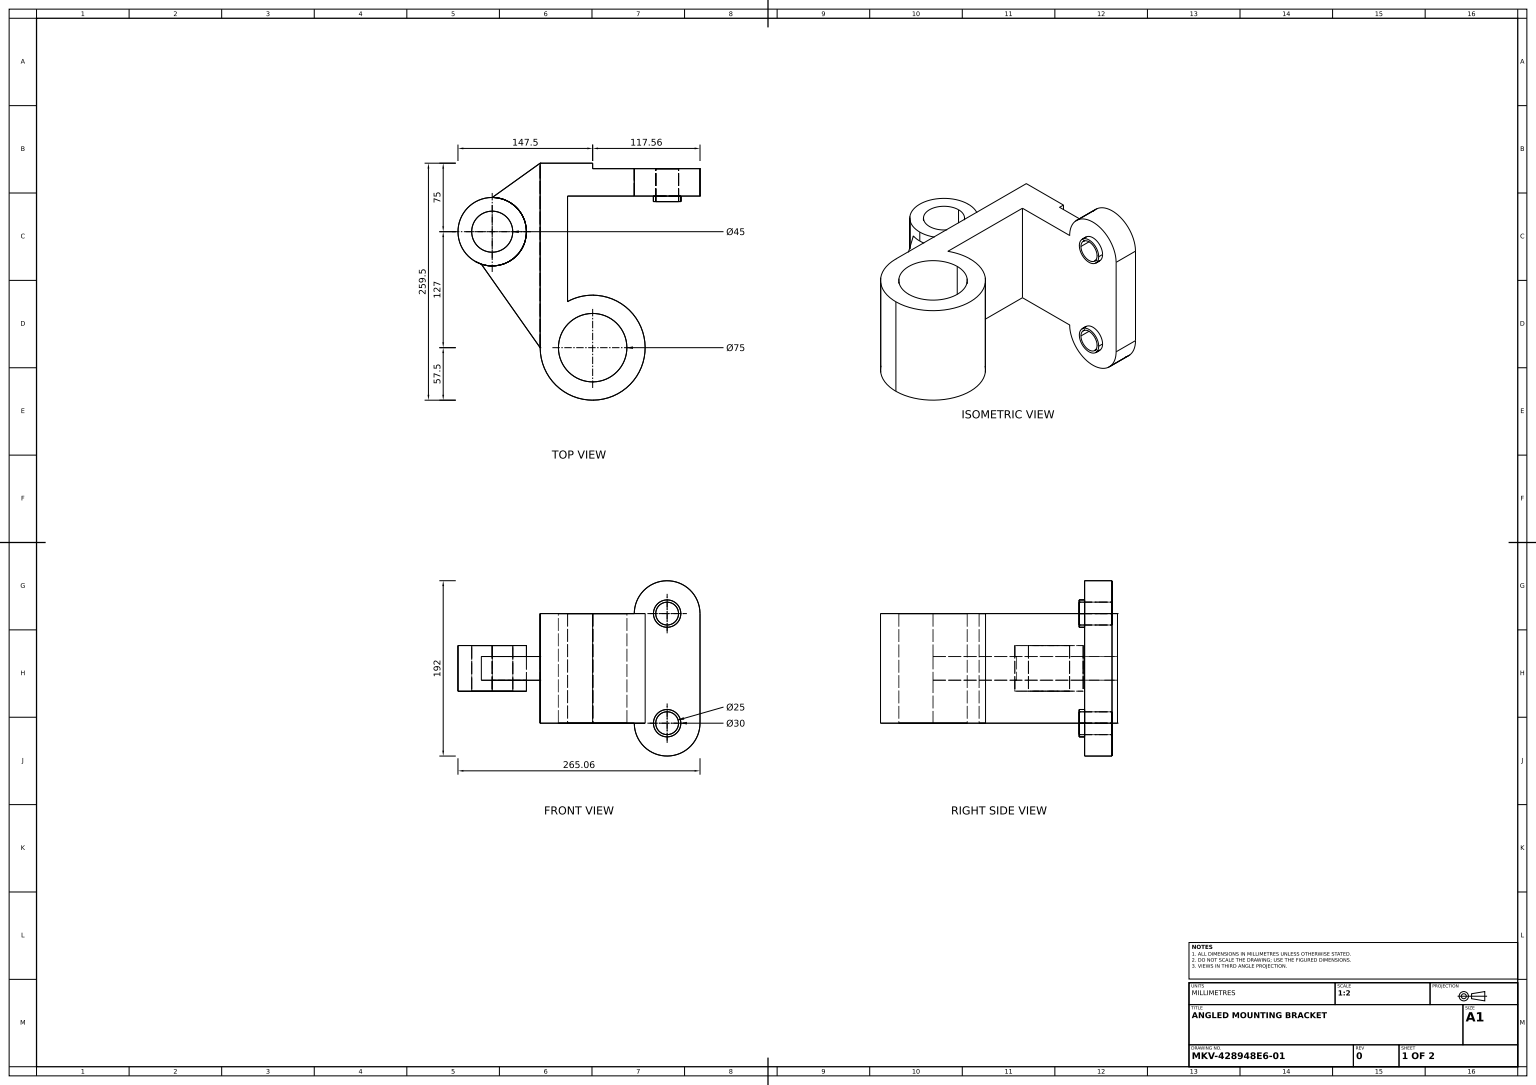
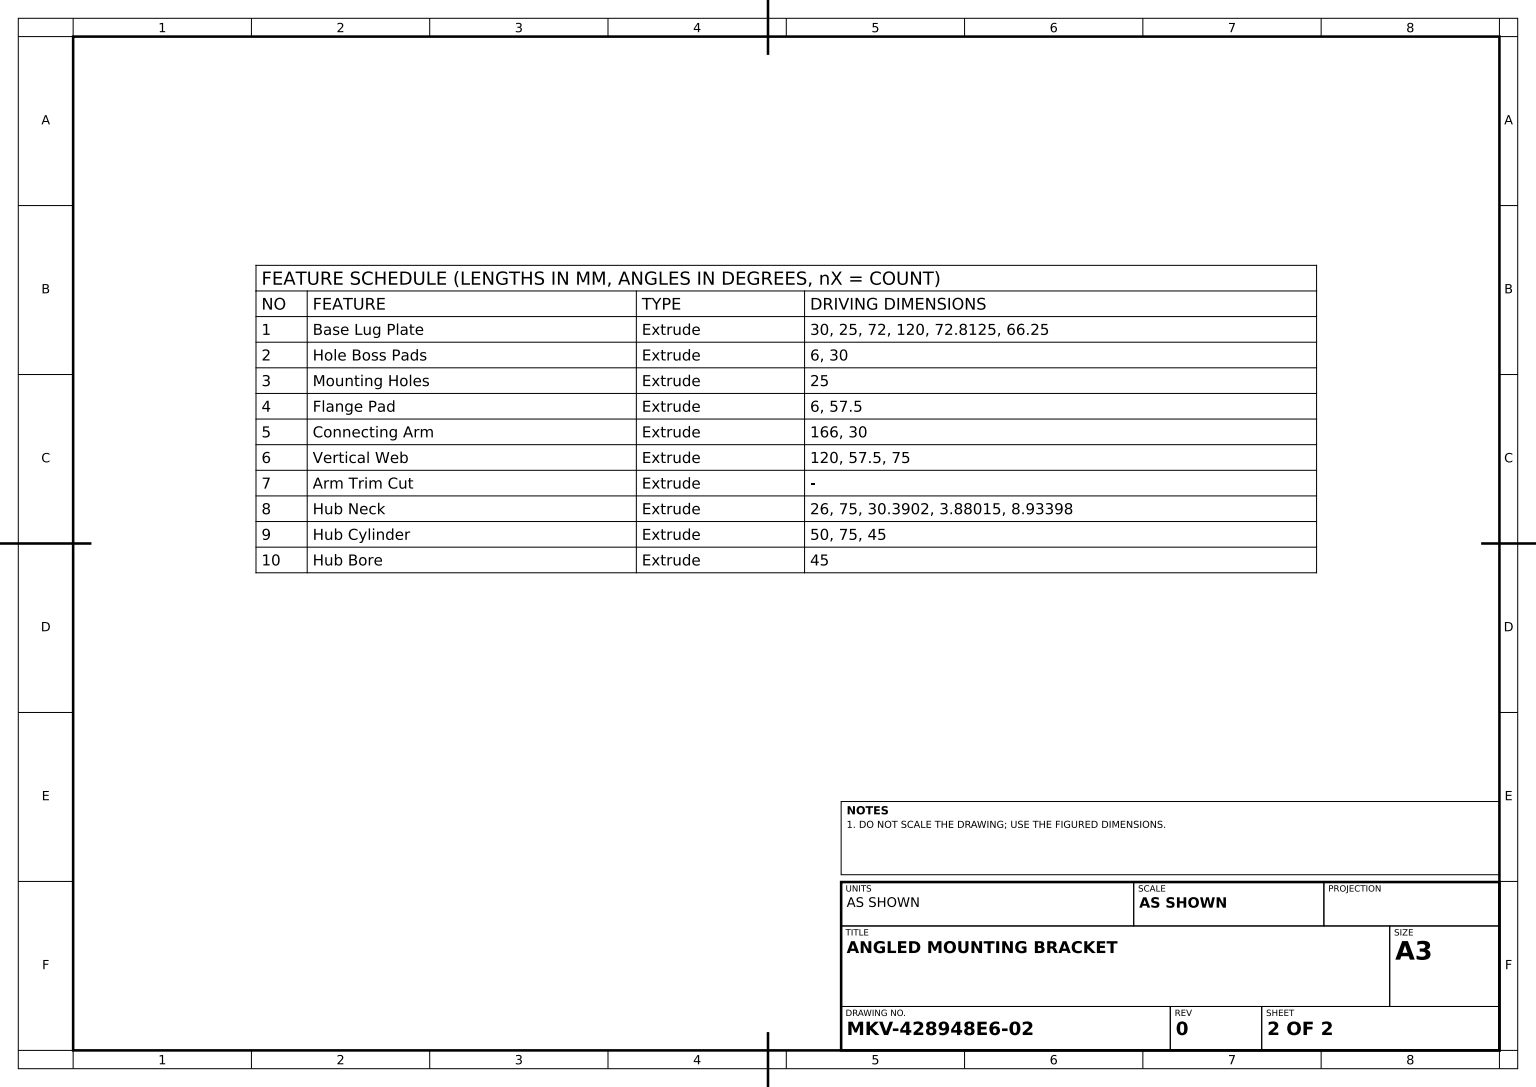
SolidWorks part; units mm, degrees
material "Plain Carbon Steel"
ref_plane "Front Plane" through (0, 0, 0) normal (0, 0, 1) x (1, 0, 0)
ref_plane "Top Plane" through (0, 0, 0) normal (0, 1, 0) x (1, 0, 0)
ref_plane "Right Plane" through (0, 0, 0) normal (1, 0, 0) x (0, 0, -1)
sketch "Base Plate Profile Sketch" plane through (0, 0, 0) normal (0, 0, 1) x (1, 0, 0)
  line L0 (0, 109.8438) -> (0, -111.7188) construction
  line L1 (-175, 0) -> (147.8125, 0) construction
  line L2 (108.8125, 60) -> (108.8125, -60)
  line L3 (36.8125, 60) -> (-66.25, 60)
  line L4 (-66.25, 60) -> (-66.25, -60)
  line L5 (-66.25, -60) -> (36.8125, -60)
  circle A0 centre (72.8125, 60) radius 12.5
  arc A1 (108.8125, 60) -> (36.8125, 60) centre (72.8125, 60) ccw
  circle A2 centre (72.8125, -60) radius 12.5
  arc A3 (36.8125, -60) -> (108.8125, -60) centre (72.8125, -60) ccw
  dimension "D1" = 25
  dimension "D2" = 72
  dimension "D3" = 25
  dimension "D4" = 72
  dimension "D5" = 120
  dimension "D6" = 72.8125
  dimension "D7" = 66.25
extrude "Base Lug Plate" add sketch "Base Plate Profile Sketch" along normal blind 30
sketch "Hole Boss Sketch" plane through (0, 0, 30) normal (0, 0, 1) x (1, 0, 0)
  circle A0 centre (72.8125, 60) radius 15
  circle A1 centre (72.8125, -60) radius 15
  dimension "D1" = 30
  dimension "D2" = 30
extrude "Hole Boss Pads" add sketch "Hole Boss Sketch" along normal blind 6
sketch "Mounting Holes Sketch" plane through (0, 0, 0) normal (0, 0, -1) x (-1, 0, 0)
  circle A0 centre (-72.8125, 60) radius 12.5
  circle A1 centre (-72.8125, -60) radius 12.5
  dimension "D1" = 25
  dimension "D2" = 25
extrude "Mounting Holes" cut sketch "Mounting Holes Sketch" against normal through all
sketch "Flange Pad Sketch" plane through (0, 0, 0) normal (0, 0, -1) x (-1, 0, 0)
  line L0 (66.25, -60) -> (-36.8125, -60) construction
  line L1 (66.25, 60) -> (8.75, 60)
  line L2 (66.25, 60) -> (66.25, -60)
  line L3 (66.25, -60) -> (8.75, -60)
  line L4 (8.75, 60) -> (8.75, -60)
  dimension "D1" = 57.5
extrude "Flange Pad" add sketch "Flange Pad Sketch" along normal blind 6 contours L2 L1 L4 L3
sketch "Connecting Arm Sketch" plane through (0, 0, 30) normal (0, 0, 1) x (1, 0, 0)
  line L0 (-66.25, 60) -> (-66.25, -60) construction
  line L1 (-66.25, 60) -> (-66.25, -60)
  line L2 (-66.25, -60) -> (36.8125, -60) construction
  line L3 (-66.25, 60) -> (-36.25, 60)
  line L4 (-66.25, 60) -> (-66.25, -60)
  line L5 (-66.25, -60) -> (-36.25, -60)
  line L6 (-36.25, 60) -> (-36.25, -60)
  line M5 (36.8125, 60) -> (-66.25, 60)
  line M6 (-66.25, 60) -> (-66.25, -60)
  line M7 (-66.25, -60) -> (36.8125, -60)
  dimension "D1" = 30
extrude "Connecting Arm" add sketch "Connecting Arm Sketch" along normal blind 166 contours L6 M5 M6 M7
sketch "Vertical Web Sketch" plane through (0, 0, 0) normal (0, 1, 0) x (1, 0, 0)
  line L0 (-66.25, -196) -> (-66.25, 6) construction
  line L1 (-66.25, -196) -> (-66.25, 6)
  line L2 (-66.25, -196) -> (-8.75, -196) construction
  circle A0 centre (-8.75, -196) radius 57.5
  circle A1 centre (-8.75, -196) radius 37.5
  dimension "D2" = 75
  dimension "D1" = 57.5
extrude "Vertical Web" add sketch "Vertical Web Sketch" along normal mid plane 120
sketch "Arm Trim Sketch" plane through (0, 60, 0) normal (0, 1, 0) x (1, 0, 0)
  line L0 (-36.25, -196) -> (-36.25, -170.5049) construction
  line L1 (-36.25, -196) -> (-36.25, -170.5049)
  line L2 (-36.25, -196) -> (-46.25, -196) construction
  line L3 (-36.25, -196) -> (-46.25, -196)
  arc A0 (-36.25, -170.5049) -> (-46.25, -196) centre (-8.75, -196) ccw
extrude "Arm Trim Cut" cut sketch "Arm Trim Sketch" against normal through all
sketch "Hub Neck Sketch" plane through (0, 0, 0) normal (0, 1, 0) x (1, 0, 0)
  line L0 (-66.25, -196) -> (-66.25, 6) construction
  line L1 (-66.25, -196) -> (-66.25, 6)
  line L2 (-66.25, -196) -> (-145.3836, -83.6359)
  line L4 (-66.25, 6) -> (-136.4497, -44.2961)
  arc A0 (-136.4497, -44.2961) -> (-141.5035, -89.1455) centre (-118.75, -69) ccw
  dimension "D2" = 30.3902
  dimension "D1" = 75
  dimension "D3" = 3.8802
  dimension "D4" = 8.934
extrude "Hub Neck" add sketch "Hub Neck Sketch" along normal mid plane 26 contours L4 A0 L2 L1
sketch "Hub Cylinder Sketch" plane through (0, 0, 0) normal (0, 1, 0) x (1, 0, 0)
  circle A0 centre (-118.75, -69) radius 37.5
  circle A1 centre (-118.75, -69) radius 22.5
  dimension "D1" = 75
  dimension "D2" = 45
extrude "Hub Cylinder" add sketch "Hub Cylinder Sketch" along normal mid plane 50
sketch "Hub Bore Sketch" plane through (0, 13, 0) normal (0, 1, 0) x (1, 0, 0)
  circle A0 centre (-118.75, -69) radius 22.5
  dimension "D1" = 45
extrude "Hub Bore" cut sketch "Hub Bore Sketch" against normal through all
